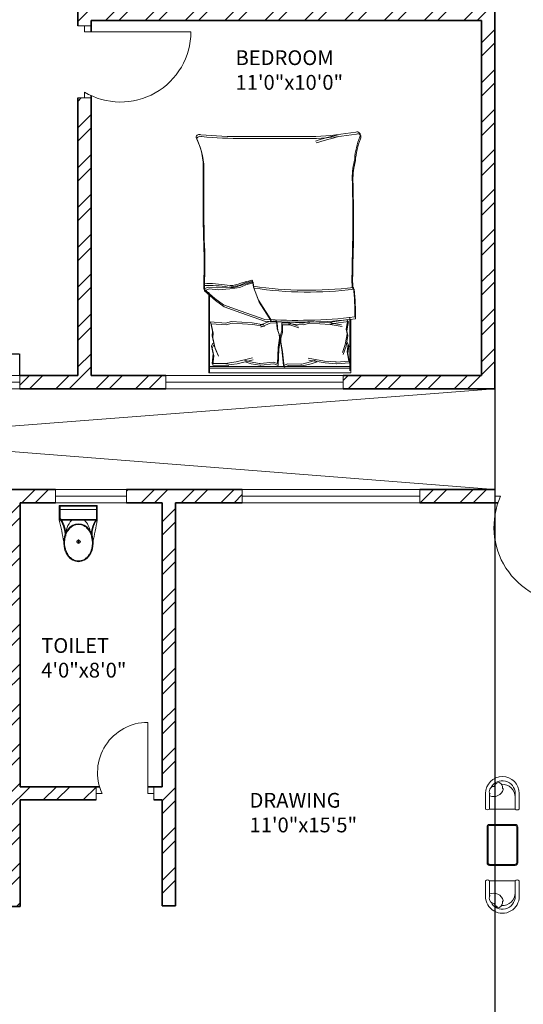
# Model space of a CAD drawing. Units: inches. Extents: x 1885 to 2748, y 783 to 2421.
# Tile 48 of 117: x 2287 to 2457, y 1350 to 1683. Entities that reach past the tile are written whole.
import ezdxf

# ---------------------------------------------------------------- set-up
doc = ezdxf.new("R2010")
doc.units = ezdxf.units.IN
for name, color, linetype, lineweight in [('A-ANNO-DIMS', 2, 'Continuous', 18), ('A-AREA-IDEN', 7, 'Continuous', 18), ('A-DOOR', 31, 'Continuous', 18), ('A-FLOR-FIXT', 8, 'Continuous', 18), ('A-FLOR-OPEN', 8, 'Continuous', 13), ('A-FURN', 8, 'Continuous', 13), ('A-GLAZ', 181, 'Continuous', 18), ('A-WALL', 7, 'Continuous', 35)]:
    doc.layers.add(name, color=color, linetype=linetype, lineweight=lineweight)
doc.layers.add('A-WALL-PATT', color=85, linetype='Continuous', lineweight=13, true_color=0x58ba48)
doc.styles.get("Standard").update_dxf_attribs({"font": 'arial.ttf'})
doc.dimstyles.get("Standard").update_dxf_attribs({"dimtxt": 0.18, "dimasz": 0.18, "dimexe": 0.18, "dimexo": 0.0625, "dimgap": 0.09, "dimtad": 0, "dimtih": 1, "dimtoh": 1, "dimdec": 4, "dimzin": 0, "dimdsep": 46, "dimtxsty": 'Standard', "dimcen": 0.09, "dimadec": 0, "dimazin": 0, "dimtfac": 1, "dimtdec": 4, "dimtofl": 0, "dimtmove": 0, "dimatfit": 3, "dimfxl": 1, "dimtolj": 1, "dimtzin": 0, "dimarcsym": 0})

# ---------------------------------------------------------------- blocks, each defined once
blk = doc.blocks.new('A$C1352')
at = {"color": 0}
for points in [[(0.003, 0.053), (0.003, 0.553, -0.414214), (0.053, 0.603), (0.753, 0.603, -0.414214), (0.803, 0.553), (0.803, 0.053, -0.414214), (0.753, 0.003), (0.053, 0.003, -0.414214)], [(0.023, 0.053), (0.023, 0.553, -0.414214), (0.053, 0.583), (0.753, 0.583, -0.414214), (0.783, 0.553), (0.783, 0.053, -0.414214), (0.753, 0.023), (0.053, 0.023, -0.414214)]]:
    blk.add_lwpolyline(points, format="xyb", close=True, dxfattribs=at)
blk = doc.blocks.new('A$C31115884')
for p, q in [((283, 498), (223, 498)), ((258, 466), (258, 523)), ((0, 200), (0, 0)), ((520, 200), (0, 200)), ((10, 190), (10, 10)), ((510, 190), (10, 190)), ((510, 10), (510, 190)), ((520, 0), (520, 200)), ((510, 54), (0, 54)), ((10, 10), (510, 10)), ((0, 0), (520, 0))]:
    blk.add_line(p, q)
blk.add_circle((256, 496), 23.6)
for centre, radius, start, end in [((2778, -205), 2807, 165.4549, 171.7133), ((-295, 403), 365, 324.2091, 9.3499), ((-295, 403), 375, 324.2091, 9.3499), ((139, 406), 293, 315.8436, 2.6563), ((806, 403), 375, 179.2036, 215.7909), ((806, 403), 365, 170.6501, 215.7909), ((3237, 905), 2807, 188.2867, 194.5451), ((384, 406), 293, 190.2774, 224.1564)]:
    blk.add_arc(centre, radius, start, end)
blk.add_ellipse((256, 510), major_axis=(0, -261), ratio=0.772727)
blk.add_open_spline([(256, 259), (263, 259), (270, 260), (288, 262), (299, 265), (320, 273), (330, 278), (350, 291), (360, 299), (378, 316), (386, 326), (402, 347), (409, 358), (421, 383), (427, 395), (436, 422), (440, 436), (445, 465), (447, 480), (448, 509), (448, 524), (445, 553), (443, 568), (436, 596), (432, 610), (422, 636), (416, 649), (402, 672), (395, 683), (379, 703), (370, 712), (351, 728), (341, 735), (321, 746), (310, 751), (289, 757), (278, 759), (256, 761), (245, 761), (223, 757), (212, 754), (191, 746), (181, 741), (161, 728), (151, 720), (133, 703), (125, 693), (110, 672), (103, 660), (90, 636), (85, 623), (76, 596), (72, 582), (67, 553), (66, 538), (64, 509), (65, 494), (68, 465), (70, 450), (77, 422), (81, 408), (91, 382), (97, 370), (111, 346), (118, 335), (135, 316), (144, 307), (162, 291), (172, 284), (193, 273), (203, 269), (225, 262), (236, 260), (250, 259), (253, 259), (256, 259)], degree=3, knots=[0, 0, 0, 0, 0.110105, 0.110105, 0.285049, 0.285049, 0.459994, 0.459994, 0.634938, 0.634938, 0.809882, 0.809882, 0.984827, 0.984827, 1.159771, 1.159771, 1.334715, 1.334715, 1.50966, 1.50966, 1.684604, 1.684604, 1.859549, 1.859549, 2.034493, 2.034493, 2.209437, 2.209437, 2.384382, 2.384382, 2.559326, 2.559326, 2.73427, 2.73427, 2.909215, 2.909215, 3.084159, 3.084159, 3.259103, 3.259103, 3.434048, 3.434048, 3.608992, 3.608992, 3.783936, 3.783936, 3.958881, 3.958881, 4.133825, 4.133825, 4.30877, 4.30877, 4.483714, 4.483714, 4.658658, 4.658658, 4.833603, 4.833603, 5.008547, 5.008547, 5.183491, 5.183491, 5.358436, 5.358436, 5.53338, 5.53338, 5.708324, 5.708324, 5.883269, 5.883269, 6.058213, 6.058213, 6.233158, 6.233158, 6.283185, 6.283185, 6.283185, 6.283185])
blk = doc.blocks.new('BED-DOUBLE')
for p, q in [((0, 51.49), (0.64, 51.49)), ((0, 3.47), (0, 51.49)), ((0, 51.26), (26.61, 51.26)), ((0, 51.26), (26.61, 51.26)), ((0.64, 51.49), (27.25, 51.49)), ((0.64, 51.49), (27.25, 51.49)), ((1.54, 3.47), (1.54, 51.26)), ((1.54, 3.47), (1.54, 51.26)), ((2.18, 3.7), (2.18, 51.49)), ((2.18, 3.7), (2.18, 51.49)), ((2.56, 50.11), (2.46, 44.71)), ((2.56, 50.11), (2.46, 44.71)), ((2.56, 50.11), (5.77, 49.73)), ((2.56, 50.11), (5.77, 49.73)), ((3.2, 50.34), (3.1, 44.94)), ((3.2, 50.34), (3.1, 44.94)), ((3.2, 50.34), (6.41, 49.96)), ((3.2, 50.34), (6.41, 49.96)), ((5.77, 49.73), (8.34, 50.33)), ((5.77, 49.73), (8.34, 50.33)), ((6.41, 49.96), (8.98, 50.56)), ((6.41, 49.96), (8.98, 50.56)), ((11.83, 50.11), (8.26, 49.31)), ((11.83, 50.11), (8.26, 49.31)), ((8.34, 50.33), (9.39, 49.81)), ((8.34, 50.33), (9.39, 49.81)), ((12.47, 50.34), (8.9, 49.54)), ((12.47, 50.34), (8.9, 49.54)), ((8.98, 50.56), (10.03, 50.04)), ((8.98, 50.56), (10.03, 50.04)), ((13.44, 49.92), (11.83, 50.11)), ((13.44, 49.92), (11.83, 50.11)), ((14.08, 50.15), (12.47, 50.34)), ((14.08, 50.15), (12.47, 50.34)), ((16.58, 50.7), (13.44, 49.92)), ((16.58, 50.7), (13.44, 49.92)), ((17.22, 50.93), (14.08, 50.15)), ((17.22, 50.93), (14.08, 50.15)), ((16.17, 45.57), (16.58, 50.7)), ((16.17, 45.56), (16.58, 50.7)), ((16.81, 45.79), (17.22, 50.93)), ((16.81, 45.79), (17.22, 50.93)), ((27.75, 52.87), (24.5, 49.16)), ((27.75, 52.87), (24.5, 49.16)), ((28.39, 53.09), (25.14, 49.39)), ((28.39, 53.09), (25.14, 49.39)), ((29.49, 52.95), (27.75, 52.87, 3.87)), ((29.49, 52.95), (27.75, 52.87, 3.87)), ((28.37, 51.33), (27.75, 52.87)), ((28.37, 51.33), (27.75, 52.87)), ((28.06, 48.23), (28.37, 51.33)), ((28.06, 48.23), (28.37, 51.33)), ((30.13, 53.17), (28.39, 53.09, 3.87)), ((30.13, 53.17), (28.39, 53.09, 3.87)), ((29.01, 51.56), (28.39, 53.09)), ((29.01, 51.56), (28.39, 53.09)), ((28.7, 48.46), (29.01, 51.56)), ((28.7, 48.46), (29.01, 51.56)), ((8.26, 49.31), (5.58, 48.13)), ((8.26, 49.31), (5.58, 48.13)), ((8.9, 49.54), (6.22, 48.36)), ((8.9, 49.54), (6.22, 48.36)), ((24.5, 49.16), (22.33, 46.22)), ((24.5, 49.16), (22.33, 46.22)), ((25.14, 49.39), (22.97, 46.45)), ((25.14, 49.39), (22.97, 46.45)), ((28.37, 44.36), (28.06, 48.23)), ((28.37, 44.36), (28.06, 48.23)), ((29.01, 44.59), (28.7, 48.46)), ((29.01, 44.59), (28.7, 48.46)), ((2.46, 44.71), (2.55, 45.71)), ((2.46, 44.71), (2.55, 45.71)), ((2.55, 45.71), (3.07, 41.91)), ((2.55, 45.71), (3.07, 41.91)), ((3.1, 44.94), (3.19, 45.94)), ((3.1, 44.94), (3.19, 45.94)), ((3.19, 45.94), (3.71, 42.14)), ((3.19, 45.94), (3.71, 42.14)), ((16.73, 43.6), (16.17, 45.57)), ((16.73, 43.6), (16.17, 45.56)), ((16.3, 36.59), (16.73, 43.6)), ((16.3, 36.59), (16.73, 43.6)), ((17.37, 43.83), (16.81, 45.79)), ((17.37, 43.83), (16.81, 45.79)), ((16.94, 36.82), (17.37, 43.83)), ((16.94, 36.82), (17.37, 43.83)), ((22.33, 46.22), (20.32, 40.64)), ((22.33, 46.22), (20.32, 40.64)), ((22.97, 46.45), (20.96, 40.87)), ((22.97, 46.45), (20.96, 40.87)), ((28.83, 40.95), (28.37, 44.36)), ((28.83, 40.95), (28.37, 44.36)), ((29.47, 41.18), (29.01, 44.59)), ((29.47, 41.18), (29.01, 44.59)), ((3.07, 41.91), (4.43, 36.49)), ((3.07, 41.91), (4.43, 36.49)), ((3.71, 42.14), (5.07, 36.72)), ((3.71, 42.14), (5.07, 36.72)), ((20.32, 40.64), (17.39, 32.3)), ((20.32, 40.64), (17.39, 32.3)), ((20.96, 40.87), (18.03, 32.53)), ((20.96, 40.87), (18.03, 32.53)), ((29.76, 38.94), (28.83, 40.95)), ((29.76, 38.94), (28.83, 40.95)), ((30.4, 39.17), (29.47, 41.18)), ((30.4, 39.17), (29.47, 41.18)), ((3.08, 37.13), (2.54, 34.2)), ((3.08, 37.13), (2.54, 34.2)), ((3.68, 39.2), (3.08, 37.13)), ((3.68, 39.2), (3.08, 37.13)), ((3.72, 37.36), (3.18, 34.43)), ((3.72, 37.36), (3.18, 34.43)), ((4.32, 39.43), (3.72, 37.36)), ((4.32, 39.43), (3.72, 37.36)), ((16.27, 32.79), (16.94, 36.82)), ((16.27, 32.79), (16.94, 36.82)), ((29.01, 36.38), (31.02, 36.69)), ((29.01, 36.38), (31.02, 36.69)), ((30.38, 36.46), (29.76, 38.94)), ((30.38, 36.46), (29.76, 38.94)), ((31.02, 36.69), (30.4, 39.17)), ((31.02, 36.69), (30.4, 39.17)), ((79.25, 15.06), (79.25, 39.68)), ((79.25, 15.06), (79.25, 39.68)), ((79.89, 15.29), (79.89, 39.9)), ((79.89, 15.29), (79.89, 39.9)), ((2.54, 34.2), (2.56, 33.88)), ((2.54, 34.2), (2.56, 33.88)), ((2.56, 33.88), (2.98, 29.45)), ((2.56, 33.88), (2.98, 29.45)), ((3.18, 34.43), (3.2, 34.11)), ((3.18, 34.43), (3.2, 34.11)), ((3.2, 34.11), (3.62, 29.68)), ((3.2, 34.11), (3.62, 29.68)), ((16.74, 30.75), (15.46, 33.82)), ((16.74, 30.75), (15.46, 33.82)), ((15.63, 32.56), (16.3, 36.59)), ((15.63, 32.56), (16.3, 36.59)), ((17.38, 30.98), (16.1, 34.05)), ((17.38, 30.98), (16.1, 34.05)), ((17.39, 30.26), (23.88, 34.45)), ((17.39, 30.26), (23.88, 34.45)), ((18.03, 30.49), (24.52, 34.68)), ((18.03, 30.49), (24.52, 34.68)), ((23.88, 34.45), (28.37, 36.15)), ((23.88, 34.45), (28.37, 36.15)), ((24.52, 34.68), (29.01, 36.38)), ((24.52, 34.68), (29.01, 36.38)), ((28.37, 36.15), (30.38, 36.46)), ((28.37, 36.15), (30.38, 36.46)), ((16.9, 28.3), (16.74, 30.75)), ((16.9, 28.3), (16.74, 30.75)), ((17.54, 28.52), (17.38, 30.98)), ((17.54, 28.52), (17.38, 30.98)), ((2.98, 29.45), (2.5, 27.98)), ((2.98, 29.45), (2.5, 27.98)), ((2.5, 27.98), (7.87, 27.73)), ((2.5, 27.98), (7.87, 27.73)), ((2.51, 26.21), (7.86, 26.79)), ((2.51, 26.21), (7.86, 26.79)), ((3.62, 29.68), (3.13, 28.2)), ((3.62, 29.68), (3.13, 28.2)), ((3.13, 28.2), (8.51, 27.96)), ((3.13, 28.2), (8.51, 27.96)), ((7.22, 26.56), (10.4, 27.14)), ((7.22, 26.56), (10.4, 27.14)), ((7.86, 26.79), (11.04, 27.37)), ((7.86, 26.79), (11.04, 27.37)), ((7.87, 27.73), (11.08, 27.35)), ((7.87, 27.73), (11.08, 27.35)), ((8.51, 27.96), (11.72, 27.58)), ((8.51, 27.96), (11.72, 27.58)), ((10.4, 27.14), (11.71, 27.14)), ((10.4, 27.14), (11.71, 27.14)), ((11.04, 27.37), (12.35, 27.37)), ((11.04, 27.37), (12.35, 27.37)), ((11.08, 27.35), (12.38, 27.43)), ((11.08, 27.35), (12.38, 27.43)), ((11.71, 27.14), (13.59, 26.56)), ((11.71, 27.14), (13.59, 26.56)), ((11.72, 27.58), (13.02, 27.66)), ((11.72, 27.58), (13.02, 27.66)), ((12.35, 27.37), (14.22, 26.79)), ((12.35, 27.37), (14.22, 26.79)), ((12.38, 27.43), (14.22, 28.13)), ((12.38, 27.43), (14.22, 28.13)), ((13.02, 27.66), (14.86, 28.36)), ((13.02, 27.66), (14.86, 28.36)), ((14.22, 28.13), (16.9, 28.3)), ((14.22, 28.13), (16.9, 28.3)), ((14.22, 26.79), (16.91, 26.79)), ((14.22, 26.79), (16.91, 26.79)), ((14.86, 28.36), (17.54, 28.52)), ((14.86, 28.36), (17.54, 28.52)), ((16.91, 26.79), (16.91, 24.33)), ((16.91, 26.79), (16.91, 24.33)), ((1.87, 25.98), (7.22, 26.56)), ((1.87, 25.98), (7.22, 26.56)), ((2.45, 24.54), (1.87, 25.98)), ((2.45, 24.54), (1.87, 25.98)), ((2.31, 20.09), (2.45, 24.54)), ((2.31, 20.09), (2.45, 24.54)), ((3.09, 24.76), (2.51, 26.21)), ((3.09, 24.76), (2.51, 26.21)), ((2.95, 20.32), (3.09, 24.76)), ((2.95, 20.32), (3.09, 24.76)), ((13.59, 26.56), (16.27, 26.56)), ((13.59, 26.56), (16.27, 26.56)), ((16.27, 24.1), (15.18, 20.96)), ((16.27, 24.1), (15.18, 20.96)), ((16.91, 24.33), (15.82, 21.19)), ((16.91, 24.33), (15.82, 21.19)), ((16.17, 19.38), (16.58, 24.51)), ((16.17, 19.38), (16.58, 24.51)), ((16.27, 26.56), (16.27, 24.1)), ((16.27, 26.56), (16.27, 24.1)), ((16.81, 19.61), (17.22, 24.74)), ((16.81, 19.61), (17.22, 24.74)), ((2.31, 19.77), (2.31, 20.09)), ((2.31, 19.77), (2.31, 20.09)), ((2.95, 20), (2.95, 20.32)), ((2.95, 20), (2.95, 20.32)), ((3.67, 17.11), (2.95, 20)), ((3.67, 17.11), (2.95, 20)), ((3.03, 16.88), (2.31, 19.77)), ((3.03, 16.88), (2.31, 19.77)), ((3.75, 14.85), (3.03, 16.88)), ((3.75, 14.85), (3.03, 16.88)), ((3.32, 12.11), (4.33, 17.6)), ((3.32, 12.11), (4.33, 17.6)), ((4.39, 15.08), (3.67, 17.11)), ((4.39, 15.08), (3.67, 17.11)), ((3.96, 12.34), (4.97, 17.83)), ((3.96, 12.34), (4.97, 17.83)), ((16.73, 17.42), (16.17, 19.38)), ((16.73, 17.42), (16.17, 19.38)), ((16.3, 10.41), (16.73, 17.42)), ((16.3, 10.41), (16.73, 17.42)), ((17.37, 17.65), (16.81, 19.61)), ((17.37, 17.65), (16.81, 19.61)), ((16.94, 10.64), (17.37, 17.65)), ((16.94, 10.64), (17.37, 17.65)), ((3.03, 8.28), (3.32, 12.11)), ((3.03, 8.28), (3.32, 12.11)), ((3.67, 8.51), (3.96, 12.34)), ((3.67, 8.51), (3.96, 12.34)), ((15.63, 6.38), (16.3, 10.41)), ((15.63, 6.38), (16.3, 10.41)), ((16.27, 6.61), (16.94, 10.64)), ((16.27, 6.61), (16.94, 10.64)), ((16.3, 10.41), (16.62, 9.28)), ((16.3, 10.41), (16.62, 9.28)), ((16.94, 10.64), (17.26, 9.51)), ((16.94, 10.64), (17.26, 9.51)), ((3.01, 8.18), (3.03, 8.28)), ((3.01, 8.18), (3.03, 8.28)), ((3.34, 3.9), (3.01, 8.18)), ((3.34, 3.9), (3.01, 8.18)), ((3.65, 8.41), (3.67, 8.51)), ((3.65, 8.41), (3.67, 8.51)), ((3.98, 4.13), (3.65, 8.41)), ((3.98, 4.13), (3.65, 8.41)), ((16.62, 9.28), (17.34, 4.18)), ((16.62, 9.28), (17.34, 4.18)), ((17.26, 9.51), (17.98, 4.41)), ((17.26, 9.51), (17.98, 4.41)), ((18.11, 3.47), (0, 3.47)), ((18.11, 3.47), (0, 3.47)), ((18.75, 3.7), (0.64, 3.7)), ((18.75, 3.7), (0.64, 3.7)), ((3.32, 3.89), (6.5, 4.47)), ((3.32, 3.89), (6.5, 4.47)), ((3.96, 4.12), (7.14, 4.7)), ((3.96, 4.12), (7.14, 4.7)), ((8.96, 5.05), (6.21, 6.06)), ((8.96, 5.05), (6.21, 6.06)), ((6.5, 4.47), (9.1, 4.04)), ((6.5, 4.47), (9.1, 4.04)), ((9.6, 5.28), (6.85, 6.29)), ((9.6, 5.28), (6.85, 6.29)), ((7.14, 4.7), (9.74, 4.27)), ((7.14, 4.7), (9.74, 4.27)), ((12.57, 4.47), (8.96, 5.05)), ((12.57, 4.47), (8.96, 5.05)), ((9.1, 4.04), (10.12, 4.62)), ((9.1, 4.04), (10.12, 4.62)), ((13.21, 4.7), (9.6, 5.28)), ((13.21, 4.7), (9.6, 5.28)), ((9.74, 4.27), (10.75, 4.84)), ((9.74, 4.27), (10.75, 4.84)), ((14.16, 4.76), (12.57, 4.47)), ((14.16, 4.76), (12.57, 4.47)), ((14.8, 4.99), (13.21, 4.7)), ((14.8, 4.99), (13.21, 4.7)), ((17.34, 4.18), (14.16, 4.76)), ((17.34, 4.18), (14.16, 4.76)), ((17.98, 4.41), (14.8, 4.99)), ((17.98, 4.41), (14.8, 4.99))]:
    blk.add_line(p, q)
for centre, radius, start, end in [((36.96, 182.49), 129.5, 266.9791, 273.8365), ((36.96, 182.49), 129.5, 266.9791, 273.8365), ((68.46, -4508.52), 4561.86, 90.00217, 90.28689), ((68.46, -4508.52), 4561.86, 90.00217, 90.28689), ((68.67, 76.16), 23.07, 267.4714, 296.4681), ((68.67, 76.16), 23.07, 267.4714, 296.4681), ((69.31, 76.38), 23.07, 267.4714, 296.4681), ((69.31, 76.38), 23.07, 267.4714, 296.4681), ((78.87, 54.41), 1.1, 332.6588, 86.02), ((78.87, 54.41), 1.1, 332.6588, 86.02), ((212.28, 41.15), 133.04, 174.4998, 180.6351), ((212.28, 41.15), 133.04, 174.4998, 180.6351), ((79.51, 54.64), 1.1, 332.6588, 86.02), ((79.51, 54.64), 1.1, 332.6588, 86.02), ((212.92, 41.38), 133.04, 174.4998, 180.6351), ((212.92, 41.38), 133.04, 174.4998, 180.6351), ((-6.65, 51.33), 36.18, 349.8763, 2.5657), ((-6.65, 51.33), 36.18, 349.8763, 2.5657), ((36.32, 182.26), 129.5, 266.9791, 273.8365), ((36.32, 182.26), 129.5, 266.9791, 273.8365), ((-6.01, 51.55), 36.18, 349.8763, 2.5657), ((-6.01, 51.55), 36.18, 349.8763, 2.5657), ((67.83, -4508.74), 4561.86, 90.00217, 90.28689), ((67.83, -4508.75), 4561.86, 90.00217, 90.28689), ((35.07, 43.74), 6.22, 168.6608, 203.7384), ((35.07, 43.74), 6.22, 168.6608, 203.7384), ((35.71, 43.97), 6.22, 168.6608, 203.7384), ((35.71, 43.97), 6.22, 168.6608, 203.7384), ((1.49, 31.15), 29.65, 10.6617, 19.8806), ((1.49, 31.15), 29.65, 10.6617, 19.8806), ((2.13, 31.38), 29.65, 10.6617, 19.8806), ((2.13, 31.38), 29.65, 10.6617, 19.8806), ((30.44, 36.64), 0.185, 250.2464, 1.1377), ((30.44, 36.63), 0.185, 250.2464, 1.1377), ((31.08, 36.86), 0.185, 250.2464, 1.1377), ((31.08, 36.86), 0.185, 250.2464, 1.1377), ((156.32, 17.75), 129.02, 171.7845, 186.9006), ((156.32, 17.75), 129.02, 171.7845, 186.9006), ((156.96, 17.98), 129.02, 171.7845, 186.9006), ((156.96, 17.98), 129.02, 171.7845, 186.9006), ((182.06, 21.36), 164.97, 176.0865, 186.7821), ((182.06, 21.36), 164.97, 176.0865, 186.7821), ((182.7, 21.59), 164.97, 176.0865, 186.7821), ((182.7, 21.59), 164.97, 176.0865, 186.7821), ((-23.71, -17.22), 106.46, 13.3832, 17.7053), ((-23.71, -17.22), 106.46, 13.3832, 17.7053), ((-23.07, -16.99), 106.46, 13.3832, 17.7053), ((-23.07, -16.99), 106.46, 13.3832, 17.7053), ((200.84, 21.43), 121.76, 182.9958, 189.4091), ((200.84, 21.43), 121.76, 182.9958, 189.4091), ((201.48, 21.65), 121.76, 182.9958, 189.4091), ((201.48, 21.65), 121.76, 182.9958, 189.4091), ((20.1, 85.16), 83.31, 268.7218, 275.604), ((20.1, 85.16), 83.31, 268.7218, 275.604), ((20.74, 85.39), 83.31, 268.7218, 275.604), ((20.74, 85.39), 83.31, 268.7218, 275.604), ((31.18, -167.31), 170.11, 88.4762, 91.0082), ((31.18, -167.31), 170.11, 88.4762, 91.0082), ((31.82, -167.08), 170.11, 88.4762, 91.0082), ((31.82, -167.08), 170.11, 88.4762, 91.0082), ((50.62, 484.82), 482.31, 268.2277, 271.7185), ((50.62, 484.82), 482.31, 268.2277, 271.7185), ((51.26, 485.05), 482.31, 268.2277, 271.7185), ((51.26, 485.05), 482.31, 268.2277, 271.7185), ((64.52, -26.9), 29.63, 76.0648, 88.9113), ((64.52, -26.9), 29.63, 76.0648, 88.9113), ((65.16, -26.67), 29.63, 76.0648, 88.9113), ((65.16, -26.67), 29.63, 76.0648, 88.9113), ((70.28, -21.66), 23.56, 67.9751, 86.652), ((70.28, -21.66), 23.56, 67.9751, 86.652), ((70.92, -21.43), 23.56, 67.9751, 86.652), ((70.92, -21.43), 23.56, 67.9751, 86.652), ((79.72, 1.09), 1.09, 236.1736, 23.4781), ((79.72, 1.09), 1.09, 236.1736, 23.4781), ((80.36, 1.31), 1.09, 236.1736, 23.4781), ((80.36, 1.31), 1.09, 236.1736, 23.4781)]:
    blk.add_arc(centre, radius, start, end)
blk = doc.blocks.new('CHAIR-LOUNGE')
blk.add_line((1.39, 5.7), (1.38, 10.98))
at = {"ltscale": 0.03}
blk.add_lwpolyline([(1.38, 10.98, 0.369229), (0, 10.98), (0, 5.7, 1), (11.42, 5.71), (11.42, 10.99, 0.369229), (10.03, 10.99)], format="xyb", close=True, dxfattribs=at)
blk.add_lwpolyline([(1.88, 3.71, 0.785087), (10.04, 5.71), (10.03, 10.99)], format="xyb")
for centre, radius, start, end in [((2.75, 3.42), 3.35, 15.7143, 112.9857), ((5.71, 6.93), 4.33, 266.342, 0.0539), ((3.01, 5.02), 1.73, 145.8599, 267.0078), ((5.71, 5.71), 4.33, 180.0539, 181.1464), ((3.98, 3.63), 1.78, 290.5305, 13.3597), ((5.79, 4.23), 0.207, 246.2577, 29.3762), ((4.77, 3.91), 1.95, 198.6466, 265.0001)]:
    blk.add_arc(centre, radius, start, end)
blk = doc.blocks.new('WIN-60')
for p, q in [((0, 60), (4.5, 60)), ((0, 60), (0, 0)), ((4.5, 60), (2.25, 60)), ((2.25, 60), (2.25, 0)), ((4.5, 0), (4.5, 60)), ((2.25, 0), (0, 0)), ((0, 0), (4.5, 0))]:
    blk.add_line(p, q)
blk = doc.blocks.new('WIN-48')
for p, q in [((0, 4.5), (0, 0)), ((48, 4.5), (0, 4.5)), ((48, 2.25), (48, 4.5)), ((48, 4.5), (48, 0)), ((0, 0), (0, 2.25)), ((0, 2.25), (48, 2.25)), ((0, 0), (48, 0))]:
    blk.add_line(p, q)
blk = doc.blocks.new('*D25')
at = {"layer": 'A-ANNO-DIMS', "color": 0, "lineweight": -2, "transparency": 16777216}
for p, q in [((2238.61, 1562.57), (2238.61, 1569.89)), ((2238.79, 1569.71), (2261.49, 1569.71)), ((2286.43, 1569.71), (2263.73, 1569.71)), ((2286.61, 1562.57), (2286.61, 1569.89))]:
    blk.add_line(p, q, dxfattribs=at)
at = {"layer": 'A-ANNO-DIMS', "color": 0, "transparency": 16777216}
for points in [[(2238.79, 1569.74), (2238.79, 1569.68), (2238.61, 1569.71)], [(2286.43, 1569.74), (2286.43, 1569.68), (2286.61, 1569.71)]]:
    blk.add_solid(points, dxfattribs=at)
at = {"layer": 'Defpoints', "color": 0, "transparency": 16777216}
for p in [(2286.61, 1569.71), (2238.61, 1562.51), (2286.61, 1562.51)]:
    blk.add_point(p, dxfattribs=at)
at = {"layer": 'A-ANNO-DIMS', "color": 0, "transparency": 16777216, "insert": (2262.61, 1569.71), "char_height": 0.18, "attachment_point": 5}
blk.add_mtext('\\A1;WINDOW 48 TYP.', dxfattribs=at)
blk = doc.blocks.new('*D55')
at = {"layer": 'A-ANNO-DIMS', "color": 0, "lineweight": -2, "transparency": 16777216}
for p, q in [((2447.27, 1557.94), (2447.27, 922.48)), ((2477.27, 1557.94), (2477.27, 922.48)), ((2447.45, 922.66), (2462.06, 922.66)), ((2477.09, 922.66), (2462.49, 922.66))]:
    blk.add_line(p, q, dxfattribs=at)
at = {"layer": 'A-ANNO-DIMS', "color": 0, "transparency": 16777216}
for points in [[(2447.45, 922.69), (2447.45, 922.63), (2447.27, 922.66)], [(2477.09, 922.69), (2477.09, 922.63), (2477.27, 922.66)]]:
    blk.add_solid(points, dxfattribs=at)
at = {"layer": 'Defpoints', "color": 0, "transparency": 16777216}
for p in [(2447.27, 1558.01), (2477.27, 1558.01), (2477.27, 922.66)]:
    blk.add_point(p, dxfattribs=at)
at = {"layer": 'A-ANNO-DIMS', "color": 0, "transparency": 16777216, "insert": (2462.27, 922.66), "char_height": 0.18, "attachment_point": 5}
blk.add_mtext('\\A1;30', dxfattribs=at)

msp = doc.modelspace()

# ---------------------------------------------------------------- hatches: boundary and pattern name
at = {"layer": 'A-WALL-PATT'}
h = msp.add_hatch(dxfattribs=at)
h.set_pattern_fill('ANSI32', color=256)
h.paths.add_polyline_path([(2007.77, 2318.01), (1980.77, 2318.01), (1980.77, 2281.22), (1985.27, 2281.22), (1985.27, 2313.51), (2007.77, 2313.51), (2007.77, 2315.76)])
h.paths.add_polyline_path([(2094.32, 2318.01), (2067.77, 2318.01), (2067.77, 2313.51), (2094.32, 2313.51), (2094.32, 2315.76)])
h.paths.add_polyline_path([(2131.37, 2315.76), (2131.37, 2318.01), (2131.19, 2318.01), (2112.61, 2318.01), (2112.61, 2313.51), (2117.27, 2313.51), (2117.27, 2255.2), (2121.77, 2255.2), (2121.77, 2313.51), (2131.37, 2313.51)])
h.paths.add_polyline_path([(2190.51, 2318.01), (2155.37, 2318.01), (2155.37, 2313.51), (2169.77, 2313.51), (2169.77, 2229.51), (2121.77, 2229.51), (2121.77, 2233.45), (2119.52, 2233.45), (2117.27, 2233.45), (2117.27, 2201.1), (2121.77, 2201.1), (2121.77, 2225.01), (2169.77, 2225.01), (2169.77, 2165.01), (2306.27, 2165.01), (2306.27, 2066.01), (2310.77, 2066.01), (2344.27, 2066.01), (2486.27, 2066.01), (2486.27, 1886.01), (2483.02, 1886.01), (2483.02, 1881.51), (2486.27, 1881.51), (2486.27, 1880.68), (2490.77, 1880.68), (2490.77, 2070.51), (2344.27, 2070.51), (2310.77, 2070.51), (2310.77, 2165.01), (2310.77, 2173.64), (2308.52, 2173.64), (2306.27, 2173.64), (2306.27, 2169.51), (2174.27, 2169.51), (2174.27, 2313.51), (2190.51, 2313.51), (2190.51, 2315.76)])
h.paths.add_polyline_path([(1985.27, 2221.22), (1980.77, 2221.22), (1980.77, 2165.01), (1992.77, 2165.01), (1992.77, 2141.93), (1997.27, 2141.93), (1997.27, 2165.01), (2117.27, 2165.01), (2117.27, 2163.13), (2121.77, 2163.13), (2121.77, 2172.73), (2119.52, 2172.73), (2117.27, 2172.73), (2117.27, 2169.51), (1985.27, 2169.51)])
h.paths.add_polyline_path([(1997.27, 2105.93), (1992.77, 2105.93), (1992.77, 2070.51), (2016.77, 2070.51), (2016.77, 2059.12), (2019.02, 2059.12), (2021.27, 2059.12), (2021.27, 2070.51), (2117.27, 2070.51), (2117.27, 2022.51), (2114.42, 2022.51), (2114.42, 2018.01), (2123.63, 2018.01), (2123.63, 2020.26), (2123.63, 2022.51), (2121.77, 2022.51), (2121.77, 2142.59), (2119.52, 2142.59), (2117.27, 2142.59), (2117.27, 2075.01), (1997.27, 2075.01)])
h.paths.add_polyline_path([(2092.03, 2020.26), (2092.03, 2022.51), (2021.27, 2022.51), (2021.27, 2035.12), (2016.77, 2035.12), (2016.77, 2018.01), (2016.77, 1978.78), (2021.27, 1978.78), (2021.27, 2018.01), (2092.03, 2018.01)])
h.paths.add_polyline_path([(2260.94, 2022.51), (2153.1, 2022.51), (2153.1, 2020.26), (2153.1, 2018.01), (2155.27, 2018.01), (2155.27, 1886.01), (2107.63, 1886.01), (2107.63, 1881.51), (2182.91, 1881.51), (2182.91, 1883.76), (2182.91, 1886.01), (2159.77, 1886.01), (2159.77, 2018.01), (2260.94, 2018.01), (2260.94, 2020.26)])
h.paths.add_polyline_path([(2047.63, 1883.76), (2047.63, 1886.01), (2021.27, 1886.01), (2021.27, 1918.78), (2019.02, 1918.78), (2016.77, 1918.78), (2016.77, 1881.51), (2047.63, 1881.51)])
h.paths.add_polyline_path([(2306.36, 1883.76), (2306.36, 1886.01), (2296.27, 1886.01), (2296.27, 1982.01), (2316.54, 1982.01), (2316.54, 1984.26), (2316.54, 1986.51), (2296.27, 1986.51), (2296.27, 2022.51), (2289.28, 2022.51), (2289.28, 2018.01), (2291.77, 2018.01), (2291.77, 1886.01), (2242.91, 1886.01), (2242.91, 1881.51), (2306.36, 1881.51)], flags=17)
h.paths.add_polyline_path([(1985.27, 1843.01), (2021.6, 1843.01), (2021.53, 1845.44), (2021.48, 1847.51), (1980.77, 1847.51), (1980.77, 1809.45), (1985.27, 1809.45)])
h.paths.add_polyline_path([(2131.48, 1845.26), (2131.48, 1847.51), (2081.53, 1847.51), (2081.53, 1843.01), (2117.27, 1843.01), (2117.27, 1784.15), (2119.52, 1784.15), (2121.77, 1784.15), (2121.77, 1843.01), (2131.48, 1843.01)])
h.paths.add_polyline_path([(2203.89, 1847.51), (2155.48, 1847.51), (2155.48, 1843.01), (2169.77, 1843.01), (2169.77, 1759.01), (2121.77, 1759.01), (2121.77, 1761.46), (2117.27, 1761.46), (2117.27, 1730.43), (2121.77, 1730.43), (2121.77, 1754.51), (2177.42, 1754.51), (2177.42, 1756.76), (2177.42, 1759.01), (2174.27, 1759.01), (2174.27, 1843.01), (2203.89, 1843.01)])
h.paths.add_polyline_path([(2335.55, 1845.26), (2335.55, 1847.51), (2239.89, 1847.51), (2239.89, 1843.01), (2306.27, 1843.01), (2306.27, 1759.01), (2199.49, 1759.01), (2199.49, 1754.51), (2310.77, 1754.51), (2310.77, 1843.01), (2335.55, 1843.01)])
h.paths.add_polyline_path([(2348.77, 2022.51), (2344.27, 2022.51), (2344.27, 1986.51), (2341.68, 1986.51), (2341.68, 1982.01), (2344.27, 1982.01), (2344.27, 1886.01), (2330.36, 1886.01), (2330.36, 1881.51), (2361.63, 1881.51), (2361.63, 1883.76), (2361.63, 1886.01), (2348.77, 1886.01)], flags=17)
h.paths.add_polyline_path([(2283.25, 2315.76), (2283.25, 2318.01), (2238.51, 2318.01), (2238.51, 2313.51), (2283.25, 2313.51)], flags=17)
h.paths.add_polyline_path([(2363.27, 2348.01), (2388.68, 2348.01), (2388.68, 2350.26), (2388.68, 2352.51), (2358.77, 2352.51), (2358.77, 2348.01), (2358.77, 2318.01), (2344.48, 2318.01), (2344.48, 2313.51), (2358.77, 2313.51), (2358.77, 2229.51), (2310.77, 2229.51), (2310.77, 2231.95), (2306.27, 2231.95), (2306.27, 2205.61), (2310.77, 2205.61), (2310.77, 2225.01), (2358.77, 2225.01), (2358.77, 2211.51), (2452.33, 2211.51), (2452.33, 2213.76), (2452.33, 2216.01), (2363.27, 2216.01), (2363.27, 2318.01)])
h.paths.add_polyline_path([(2310.77, 2313.51), (2320.48, 2313.51), (2320.48, 2315.76), (2320.48, 2318.01), (2302.73, 2318.01), (2302.73, 2313.51), (2306.27, 2313.51), (2306.27, 2251.08), (2310.77, 2251.08)], flags=17)
h.paths.add_polyline_path([(2490.77, 2352.51), (2486.27, 2352.51), (2448.68, 2352.51), (2448.68, 2348.01), (2486.27, 2348.01), (2486.27, 2318.01), (2486.27, 2216.01), (2481.78, 2216.01), (2481.78, 2211.51), (2486.27, 2211.51), (2486.27, 2165.01), (2493.29, 2165.01), (2493.29, 2167.26), (2493.29, 2169.51), (2490.77, 2169.51), (2490.77, 2313.51), (2494.43, 2313.51), (2494.43, 2318.01), (2490.77, 2318.01)])
h.paths.add_polyline_path([(2534.65, 2318.01), (2515.69, 2318.01), (2515.69, 2313.51), (2534.65, 2313.51), (2534.65, 2315.76)])
h.paths.add_polyline_path([(2618.27, 2318.01), (2594.65, 2318.01), (2594.65, 2313.51), (2613.77, 2313.51), (2613.77, 2281.71), (2618.27, 2281.71)])
h.paths.add_polyline_path([(2618.27, 2221.71), (2613.77, 2221.71), (2613.77, 2169.51), (2554.02, 2169.51), (2554.02, 2165.01), (2613.77, 2165.01), (2613.77, 2152.88), (2618.27, 2152.88)])
h.paths.add_polyline_path([(2618.27, 2128.88), (2616.02, 2128.88), (2613.77, 2128.88), (2613.77, 2117.01), (2529.77, 2117.01), (2529.77, 2165.01), (2532.85, 2165.01), (2532.85, 2169.51), (2522.87, 2169.51), (2522.87, 2165.01), (2525.27, 2165.01), (2525.27, 2117.01), (2525.27, 2112.51), (2525.27, 2108.58), (2529.77, 2108.58), (2529.77, 2112.51), (2613.77, 2112.51), (2613.77, 2080.19), (2618.27, 2080.19)])
h.paths.add_polyline_path([(2618.27, 2044.19), (2616.02, 2044.19), (2613.77, 2044.19), (2613.77, 2015.51), (2529.77, 2015.51), (2529.77, 2088.58), (2527.52, 2088.58), (2525.27, 2088.58), (2525.27, 2011.01), (2613.77, 2011.01), (2613.77, 1956.75), (2618.27, 1956.75)])
h.paths.add_polyline_path([(2618.27, 1881.51), (2618.27, 1896.75), (2613.77, 1896.75), (2613.77, 1881.51), (2613.77, 1847.51), (2592.71, 1847.51), (2592.71, 1843.01), (2613.77, 1843.01), (2613.77, 1765.01), (2613.77, 1760.51), (2609.62, 1760.51), (2609.62, 1756.01), (2613.77, 1756.01), (2613.77, 1660.01), (2608.54, 1660.01), (2608.54, 1655.51), (2613.77, 1655.51), (2613.77, 1508.16), (2618.27, 1508.16)])
h.paths.add_polyline_path([(2565.77, 1843.01), (2569, 1843.01), (2569, 1847.51), (2490.77, 1847.51), (2490.77, 1849.7), (2488.52, 1849.7), (2486.27, 1849.7), (2486.27, 1847.51), (2477.27, 1847.51), (2477.27, 1838.51), (2477.27, 1821.49), (2486.27, 1821.49), (2486.27, 1838.51), (2561.27, 1838.51), (2561.27, 1765.01), (2486.27, 1765.01), (2486.27, 1786.16), (2477.27, 1786.16), (2477.27, 1765.01), (2477.27, 1756.01), (2486.27, 1756.01), (2565.77, 1756.01), (2585.62, 1756.01), (2585.62, 1758.26), (2585.62, 1760.51), (2565.77, 1760.51), (2565.77, 1765.01)])
h.paths.add_polyline_path([(2486.27, 1651.01), (2561.27, 1651.01), (2561.27, 1567.01), (2486.27, 1567.01), (2486.27, 1591.32), (2477.27, 1591.32), (2477.27, 1567.01), (2477.27, 1558.01), (2477.27, 1555.44), (2481.77, 1555.44), (2481.77, 1558.01), (2568.65, 1558.01), (2568.65, 1560.26), (2568.65, 1562.51), (2565.77, 1562.51), (2565.77, 1655.51), (2584.54, 1655.51), (2584.54, 1657.76), (2584.54, 1660.01), (2565.77, 1660.01), (2486.27, 1660.01), (2477.27, 1660.01), (2477.27, 1651.01), (2477.27, 1632.99), (2486.27, 1632.99)])
h.paths.add_polyline_path([(2449.97, 1883.76), (2449.97, 1886.01), (2421.63, 1886.01), (2421.63, 1881.51), (2449.97, 1881.51)], flags=17)
h.paths.add_polyline_path([(2447.27, 1847.51), (2395.55, 1847.51), (2395.55, 1843.01), (2442.77, 1843.01), (2442.77, 1809.27), (2447.27, 1809.27)])
h.paths.add_polyline_path([(1985.27, 1749.45), (1980.77, 1749.45), (1980.77, 1694.5), (1985.27, 1694.5), (1985.27, 1694.51), (1986.9, 1694.51), (1986.9, 1697.78), (1986.9, 1699.01), (1985.27, 1699.01)])
h.paths.add_polyline_path([(2152.77, 1699.01), (2121.77, 1699.01), (2121.77, 1703.67), (2119.52, 1703.67), (2117.27, 1703.67), (2117.27, 1699.01), (2009.22, 1699.01), (2009.22, 1694.51), (2148.27, 1694.51), (2148.27, 1692.63), (2152.77, 1692.63)])
h.paths.add_polyline_path([(2016.27, 1694.51), (2011.77, 1694.51), (2011.77, 1558.01), (2040.81, 1558.01), (2040.81, 1560.26), (2040.81, 1562.51), (2016.27, 1562.51)])
h.paths.add_polyline_path([(2152.77, 1663.02), (2150.52, 1663.02), (2148.27, 1663.02), (2148.27, 1562.51), (2100.81, 1562.51), (2100.81, 1558.01), (2165.12, 1558.01), (2165.12, 1560.26), (2165.12, 1562.51), (2152.77, 1562.51), (2152.77, 1610.51), (2224.77, 1610.51), (2224.77, 1607.99), (2229.27, 1607.99), (2229.27, 1615.01), (2152.77, 1615.01)])
h.paths.add_polyline_path([(2238.61, 1560.26), (2238.61, 1562.51), (2229.27, 1562.51), (2229.27, 1588.76), (2227.02, 1588.76), (2224.77, 1588.77), (2224.77, 1562.51), (2189.12, 1562.51), (2189.12, 1558.01), (2238.61, 1558.01)])
h.paths.add_polyline_path([(2336.02, 1560.26), (2336.02, 1562.51), (2310.77, 1562.51), (2310.77, 1656.35), (2308.52, 1656.35), (2306.27, 1656.35), (2306.27, 1562.51), (2286.61, 1562.51), (2286.61, 1558.01), (2336.02, 1558.01)])
h.paths.add_polyline_path([(2447.27, 1690.97), (2445.02, 1690.97), (2442.77, 1690.97), (2442.77, 1687.01), (2306.27, 1687.01), (2306.27, 1680.75), (2310.77, 1680.75), (2310.77, 1682.51), (2442.77, 1682.51), (2442.77, 1562.51), (2396.02, 1562.51), (2396.02, 1558.01), (2447.27, 1558.01)])
h.paths.add_polyline_path([(2447.27, 1749.27), (2445.02, 1749.27), (2442.77, 1749.27), (2442.77, 1717.23), (2447.27, 1717.23)])
h.paths.add_polyline_path([(2044.67, 1521.76), (2044.67, 1524.01), (2007.27, 1524.01), (2007.27, 1503.49), (2009.52, 1503.49), (2011.77, 1503.49), (2011.77, 1519.51), (2044.67, 1519.51)])
h.paths.add_polyline_path([(2177.97, 1521.76), (2177.97, 1524.01), (2104.67, 1524.01), (2104.67, 1519.51), (2145.77, 1519.51), (2145.77, 1387.51), (2143.37, 1387.51), (2143.37, 1383.01), (2251.59, 1383.01), (2251.59, 1385.26), (2251.59, 1387.51), (2150.27, 1387.51), (2150.27, 1519.51), (2177.97, 1519.51)])
h.paths.add_polyline_path([(2298.7, 1524.01), (2237.97, 1524.01), (2237.97, 1519.51), (2282.27, 1519.51), (2282.27, 1387.51), (2279.68, 1387.51), (2279.68, 1383.01), (2286.77, 1383.01), (2286.77, 1419.01), (2312.45, 1419.01), (2312.45, 1421.26), (2312.45, 1423.51), (2286.77, 1423.51), (2286.77, 1519.51), (2298.7, 1519.51), (2298.7, 1521.72)], flags=17)
h.paths.add_polyline_path([(2361.9, 1521.76), (2361.9, 1524.01), (2322.7, 1524.01), (2322.7, 1519.51), (2334.77, 1519.51), (2334.77, 1423.51), (2331.93, 1423.51), (2331.93, 1419.01), (2334.77, 1419.01), (2334.77, 1387.51), (2334.77, 1383.23), (2339.27, 1383.23), (2339.27, 1387.51), (2339.27, 1519.51), (2361.9, 1519.51)], flags=17)
h.paths.add_polyline_path([(2447.27, 1521.76), (2447.27, 1524.01), (2421.9, 1524.01), (2421.9, 1519.51), (2447.27, 1519.51)], flags=17)
h.paths.add_polyline_path([(2481.77, 1529.6), (2479.52, 1529.6), (2477.27, 1529.6), (2477.27, 1524.01), (2474.49, 1524.01), (2474.49, 1519.51), (2477.27, 1519.51), (2477.27, 1334.51), (2296.77, 1334.51), (2296.77, 1240.51), (2160.27, 1240.51), (2160.27, 1180.51), (2112.27, 1180.51), (2112.27, 1207.69), (2110.02, 1207.69), (2107.77, 1207.69), (2107.77, 1171.61), (2112.27, 1171.61), (2112.27, 1176.01), (2160.27, 1176.01), (2160.27, 1092.01), (2144.22, 1092.01), (2144.22, 1087.51), (2189.5, 1087.51), (2189.5, 1089.76), (2189.5, 1092.01), (2164.77, 1092.01), (2164.77, 1236.01), (2296.77, 1236.01), (2296.77, 1231.91), (2301.27, 1231.91), (2301.27, 1330.01), (2481.77, 1330.01), (2481.77, 1387.51)])
h.paths.add_polyline_path([(2618.27, 1448.16), (2613.77, 1448.16), (2613.77, 1382.51), (2529.77, 1382.51), (2525.27, 1382.51), (2525.27, 1307.06), (2529.77, 1307.06), (2529.77, 1378.01), (2613.77, 1378.01), (2613.77, 1354.99), (2618.27, 1354.99)])
h.paths.add_polyline_path([(2618.27, 1318.99), (2613.77, 1318.99), (2613.77, 1281.01), (2529.77, 1281.01), (2529.77, 1283.79), (2527.52, 1283.79), (2525.27, 1283.79), (2525.27, 1228.51), (2516.79, 1228.51), (2516.79, 1224.01), (2533.48, 1224.01), (2533.48, 1226.26), (2533.48, 1228.51), (2529.77, 1228.51), (2529.77, 1276.51), (2613.77, 1276.51), (2613.77, 1266.02), (2618.27, 1266.02)])
h.paths.add_polyline_path([(2618.27, 1134.96), (2613.77, 1134.96), (2613.77, 1092.01), (2594.54, 1092.01), (2594.54, 1087.51), (2618.27, 1087.51)])
h.paths.add_polyline_path([(2534.54, 1092.01), (2509.77, 1092.01), (2509.77, 1087.51), (2534.54, 1087.51), (2534.54, 1089.76)])
h.paths.add_polyline_path([(2481.27, 1224.01), (2484.12, 1224.01), (2484.12, 1226.26), (2484.12, 1228.51), (2476.77, 1228.51), (2476.77, 1198.51), (2471.61, 1198.51), (2471.61, 1194.01), (2476.77, 1194.01), (2476.77, 1062.01), (2436.89, 1062.01), (2436.89, 1057.51), (2476.77, 1057.51), (2481.27, 1057.51), (2481.27, 1062.01), (2481.27, 1087.51), (2485.35, 1087.51), (2485.35, 1089.76), (2485.35, 1092.01), (2481.27, 1092.01), (2481.27, 1117.51)])
h.paths.add_polyline_path([(2439.9, 1198.51), (2349.27, 1198.51), (2349.27, 1194.01), (2349.27, 1180.51), (2301.27, 1180.51), (2301.27, 1201.9), (2299.02, 1201.9), (2296.77, 1201.9), (2296.77, 1172.34), (2299.02, 1172.34), (2301.27, 1172.34), (2301.27, 1176.01), (2349.27, 1176.01), (2349.27, 1092.01), (2334.45, 1092.01), (2334.45, 1087.51), (2349.27, 1087.51), (2349.27, 1057.51), (2353.77, 1057.51), (2376.89, 1057.51), (2376.89, 1059.76), (2376.89, 1062.01), (2353.77, 1062.01), (2353.77, 1087.51), (2353.77, 1180.51), (2353.77, 1194.01), (2439.9, 1194.01), (2439.9, 1196.26)])
h.paths.add_polyline_path([(2270.6, 1089.76), (2270.6, 1092.01), (2249.5, 1092.01), (2249.5, 1087.51), (2270.6, 1087.51)], flags=17)
h.paths.add_polyline_path([(2310.45, 1092.01), (2301.27, 1092.01), (2301.27, 1153.29), (2296.77, 1153.29), (2296.77, 1092.01), (2293.79, 1092.01), (2293.79, 1087.51), (2310.45, 1087.51), (2310.45, 1089.76)], flags=17)
h.paths.add_polyline_path([(2112.27, 1150.33), (2110.02, 1150.33), (2107.77, 1150.33), (2107.77, 1092.01), (2104.47, 1092.01), (2104.47, 1087.51), (2120.22, 1087.51), (2120.22, 1089.76), (2120.22, 1092.01), (2112.27, 1092.01)])
h.paths.add_polyline_path([(2082.17, 1092.01), (2058.14, 1092.01), (2058.14, 1087.51), (2082.17, 1087.51), (2082.17, 1089.76)])
h.paths.add_polyline_path([(1975.77, 1145.64), (1971.27, 1145.64), (1971.27, 1087.51), (1980.77, 1087.51), (1998.14, 1087.51), (1998.14, 1089.76), (1998.14, 1092.01), (1985.27, 1092.01), (1975.77, 1092.01)])
h.paths.add_polyline_path([(2112.27, 1244.38), (2110.02, 1244.38), (2107.77, 1244.38), (2107.77, 1240.51), (1992.27, 1240.51), (1992.27, 1271.01), (1987.77, 1271.01), (1987.77, 1240.51), (1980.77, 1240.51), (1975.77, 1240.51), (1971.27, 1240.51), (1971.27, 1205.64), (1975.77, 1205.64), (1975.77, 1236.01), (2107.77, 1236.01), (2107.77, 1233.44), (2112.27, 1233.44), (2112.27, 1236.01)])
h.paths.add_polyline_path([(2112.27, 1383.01), (2114.78, 1383.01), (2114.78, 1385.26), (2114.78, 1387.51), (2102.48, 1387.51), (2102.48, 1383.01), (2107.77, 1383.01), (2107.77, 1335.01), (2011.77, 1335.01), (2011.77, 1349.94), (2007.27, 1349.94), (2007.27, 1335.01), (1987.77, 1335.01), (1987.77, 1330.51), (1987.77, 1307.01), (1992.27, 1307.01), (1992.27, 1330.51), (2007.27, 1330.51), (2107.77, 1330.51), (2107.77, 1264.71), (2112.27, 1264.71)])
h.paths.add_polyline_path([(2077.86, 1387.51), (2011.77, 1387.51), (2011.77, 1390.04), (2009.52, 1390.04), (2007.27, 1390.04), (2007.27, 1373.94), (2011.77, 1373.94), (2011.77, 1383.01), (2077.86, 1383.01)])
h.paths.add_polyline_path([(2011.77, 1443.49), (2007.27, 1443.49), (2007.27, 1410.25), (2011.77, 1410.25)])

# ---------------------------------------------------------------- linework, layer by layer
at = {"layer": 'A-DOOR'}
for p, q in [((2306.27, 1680.75), (2310.77, 1680.75)), ((2310.77, 1680.75), (2308.52, 1680.75)), ((2308.52, 1680.75), (2308.52, 1678.75)), ((2308.52, 1678.75), (2344.52, 1678.75)), ((2308.52, 1656.35), (2308.52, 1658.35)), ((2306.27, 1656.35), (2310.77, 1656.35)), ((2310.77, 1656.35), (2308.52, 1656.35)), ((2447.27, 1524.01), (2447.27, 1519.51)), ((2447.27, 1519.51), (2447.27, 1521.76)), ((2447.27, 1521.76), (2449.27, 1521.76)), ((2329.93, 1421.26), (2329.93, 1445.26)), ((2312.45, 1423.51), (2312.45, 1419.01)), ((2331.93, 1423.51), (2331.93, 1419.01)), ((2312.45, 1419.01), (2312.45, 1421.26)), ((2312.45, 1421.26), (2314.45, 1421.26)), ((2331.93, 1421.26), (2329.93, 1421.26)), ((2331.93, 1419.01), (2331.93, 1421.26))]:
    msp.add_line(p, q, dxfattribs=at)
for centre, radius, start, end in [((2320.74, 1678.75), 23.78, 239.0847, 0), ((2472.49, 1511.24), 25.49, 155.6331, 270), ((2329.93, 1428.26), 16.99, 90, 204.3606)]:
    msp.add_arc(centre, radius, start, end, dxfattribs=at)
at = {"layer": 'A-FLOR-OPEN'}
for p, q in [((2007.27, 1524.01), (2447.27, 1558.01)), ((2447.27, 1524.01), (2011.77, 1558.01)), ((2447.27, 1558.01), (2447.27, 1524.01))]:
    msp.add_line(p, q, dxfattribs=at)
at = {"layer": 'A-GLAZ'}
for p, q in [((2298.7, 1524.01), (2298.7, 1520.15)), ((2298.7, 1524.01), (2322.7, 1524.01)), ((2298.7, 1519.51), (2298.7, 1521.72)), ((2298.7, 1521.72), (2322.7, 1521.72)), ((2322.7, 1521.72), (2322.7, 1524.01)), ((2322.7, 1524.01), (2322.7, 1519.51)), ((2298.7, 1520.15), (2298.7, 1519.51)), ((2322.7, 1519.51), (2298.7, 1519.51))]:
    msp.add_line(p, q, dxfattribs=at)
at = {"layer": 'A-WALL'}
for p, q in [((2447.27, 1690.97), (2447.27, 1558.01)), ((2306.27, 1687.01), (2306.27, 1680.75)), ((2310.77, 1682.51), (2442.77, 1682.51)), ((2310.77, 1682.51), (2310.77, 1678.75)), ((2442.77, 1682.51), (2442.77, 1562.51)), ((2306.27, 1656.35), (2306.27, 1562.51)), ((2310.77, 1657.16), (2310.77, 1562.51)), ((2286.61, 1562.51), (2306.27, 1562.51)), ((2310.77, 1562.51), (2336.02, 1562.51)), ((2396.02, 1562.51), (2442.77, 1562.51)), ((2286.61, 1558.01), (2336.02, 1558.01)), ((2396.02, 1558.01), (2447.27, 1558.01)), ((2237.97, 1524.01), (2298.7, 1524.01)), ((2322.7, 1524.01), (2361.9, 1524.01)), ((2421.9, 1524.01), (2447.27, 1524.01)), ((2286.77, 1519.51), (2286.77, 1423.51)), ((2286.77, 1519.51), (2298.7, 1519.51)), ((2322.7, 1519.51), (2334.77, 1519.51)), ((2334.77, 1519.51), (2334.77, 1423.51)), ((2339.27, 1519.51), (2339.27, 1387.51)), ((2339.27, 1519.51), (2361.9, 1519.51)), ((2421.9, 1519.51), (2448.38, 1519.51)), ((2286.77, 1423.51), (2313.62, 1423.51)), ((2329.93, 1423.51), (2334.77, 1423.51)), ((2286.77, 1419.01), (2312.45, 1419.01)), ((2286.77, 1419.01), (2286.77, 1383.01)), ((2331.93, 1419.01), (2334.77, 1419.01)), ((2334.77, 1419.01), (2334.77, 1387.51)), ((2334.77, 1387.51), (2334.77, 1383.23)), ((2339.27, 1383.23), (2339.27, 1387.51)), ((2286.77, 1383.01), (2279.68, 1383.01)), ((2334.77, 1383.23), (2339.27, 1383.23))]:
    msp.add_line(p, q, dxfattribs=at)

# ---------------------------------------------------------------- block references
at = {"layer": 'A-FLOR-FIXT', "xscale": 0.0246256636748975, "yscale": 0.0246256636748975, "zscale": 0.0246256636748975, "rotation": 180}
msp.add_blockref('A$C31115884', (2312.81, 1518.56), dxfattribs=at)
at = {"layer": 'A-FURN', "rotation": 89.99999983318565}
msp.add_blockref('BED-DOUBLE', (2402.02, 1563.43), dxfattribs=at)
at = {"layer": 'A-FURN', "extrusion": (0, 0, -1), "zscale": -1, "rotation": 180}
msp.add_blockref('CHAIR-LOUNGE', (-2444.15, 1426.92), dxfattribs=at)
at = {"layer": 'A-FURN', "ltscale": 0.03, "xscale": 17.30251319894821, "yscale": 17.30251319894821, "zscale": 17.30251319894821, "rotation": 270}
msp.add_blockref('A$C1352', (2444.62, 1410.79), dxfattribs=at)
at = {"layer": 'A-FURN'}
msp.add_blockref('CHAIR-LOUNGE', (2444.15, 1380.73), dxfattribs=at)
at = {"layer": 'A-GLAZ'}
msp.add_blockref('WIN-48', (2238.61, 1558.01), dxfattribs=at)
at = {"layer": 'A-GLAZ', "extrusion": (0, 0, -1), "zscale": -1, "rotation": 90}
for p in [(-2336.03, 1558), (-2361.9, 1519.5)]:
    msp.add_blockref('WIN-60', p, dxfattribs=at)

# ---------------------------------------------------------------- texts
at = {"layer": 'A-AREA-IDEN', "char_height": 5, "attachment_point": 1}
for s, width, insert in [('BEDROOM\\P11\'0"x10\'0"', 110.4323, (2359.61, 1672.46)), ('TOILET\\P4\'0"x8\'0"', 133.5219, (2293.9, 1473.74)), ('DRAWING\\P11\'0"x15\'5"', 189.8784, (2364.35, 1421.41))]:
    msp.add_mtext_dynamic_manual_height_columns(s, width=width, gutter_width=12.5, heights=[0], dxfattribs=dict(at, insert=insert))

# ---------------------------------------------------------------- dimensions: what is measured, and where the dimension line sits
at = {"layer": 'A-ANNO-DIMS'}
dim = msp.add_linear_dim(base=(2286.61, 1569.71), p1=(2238.61, 1562.51), p2=(2286.61, 1562.51), text='WINDOW <> TYP.', dimstyle='Standard', override={"dimdec": 0, "dimlfac": 1, "dimrnd": 0, "dimzin": 0, "dimdsep": 46, "dimlunit": 2}, dxfattribs=at)
dim.commit()
dim.dimension.update_dxf_attribs({"geometry": '*D25', "text_midpoint": (2262.61, 1569.71)})
dim = msp.add_linear_dim(base=(2477.27, 922.66), p1=(2447.27, 1558.01), p2=(2477.27, 1558.01), dimstyle='Standard', override={"dimdec": 0, "dimlfac": 1, "dimrnd": 0, "dimzin": 0, "dimdsep": 46, "dimlunit": 2}, dxfattribs=at)
dim.commit()
dim.dimension.update_dxf_attribs({"geometry": '*D55', "text_midpoint": (2462.27, 922.66)})

doc.saveas('drawing.dxf')
